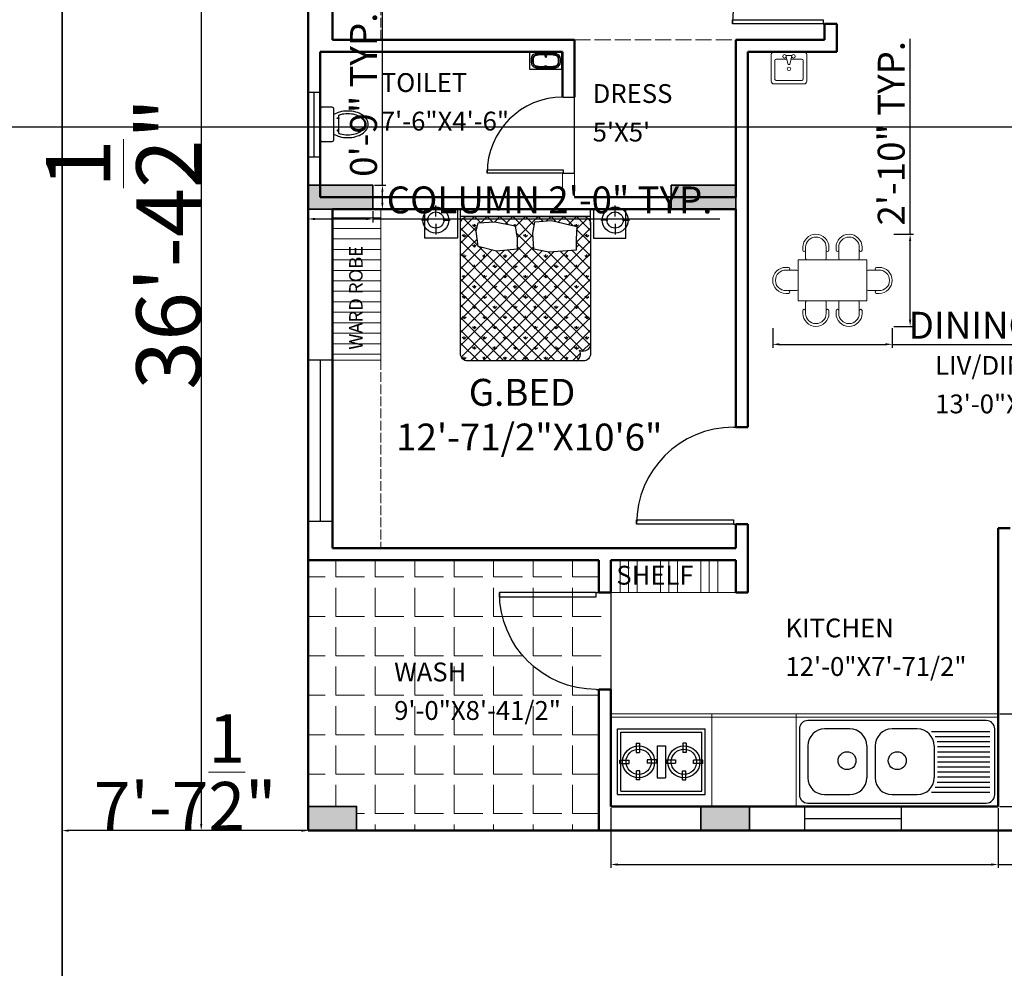
# Model space of a CAD drawing. Units: inches. Extents: x 2214 to 3937, y 762 to 2085.
# Tile 3 of 9: x 2567 to 2933, y 1424 to 1777. Entities that reach past the tile are written whole.
import ezdxf

# ---------------------------------------------------------------- set-up
doc = ezdxf.new("R2010")
doc.units = ezdxf.units.IN
doc.linetypes.add('ACAD_ISO02W100', pattern=[15, 12, -3])
for name, color, linetype, lineweight in [('A-ANNO-DIMS', 2, 'Continuous', 18), ('A-ANNO-TEXT', 7, 'Continuous', 18), ('A-AREA-IDEN', 7, 'Continuous', 25), ('A-CASE', 252, 'Continuous', 18), ('A-CASE-OVHD', 252, 'ACAD_ISO02W100', 13), ('A-CASE-PATT', 252, 'Continuous', 13), ('A-COLS', 5, 'Continuous', 35), ('A-FLOR-FIXT', 9, 'Continuous', 18), ('A-FLOR-PATT', 116, 'Continuous', 13), ('A-FURN', 8, 'Continuous', 18), ('A-WALL-OVHD', 20, 'ACAD_ISO02W100', 18), ('C-ANNO-DIMS', 2, 'Continuous', 18), ('C-PROP', 3, 'Continuous', 35), ('door', 122, 'Continuous', 25), ('wall', 20, 'Continuous', 50), ('wardrobe', 252, 'Continuous', 18), ('window', 4, 'Continuous', 25)]:
    doc.layers.add(name, color=color, linetype=linetype, lineweight=lineweight)
for name, color, linetype in [('GIUONG', 70, 'Continuous'), ('NOI THAT', 42, 'Continuous'), ('THIET-BI', 21, 'Continuous')]:
    doc.layers.add(name, color=color, linetype=linetype)
doc.styles.add('ATT', font='romans.shx')
doc.styles.get("Standard").update_dxf_attribs({"font": 'arial.ttf'})
doc.dimstyles.new('ISO-25', dxfattribs={"dimtxt": 10, "dimasz": 2.5, "dimexe": 1.25, "dimexo": 0.625, "dimtad": 1, "dimdec": 1, "dimlunit": 4, "dimtxsty": 'Standard', "dimcen": 2.5, "dimadec": 0, "dimazin": 0, "dimtfac": 1, "dimtdec": 1, "dimtmove": 0, "dimatfit": 3, "dimfxl": 1, "dimarcsym": 0})

# ---------------------------------------------------------------- blocks, each defined once
blk = doc.blocks.new('*U2')
for p, q in [((0, 0), (0, -6)), ((40, 0), (40, -6))]:
    blk.add_line(p, q)
blk.add_lwpolyline([(0, 0), (0, 40), (1.75, 40), (1.75, 0)], close=True)
blk.add_arc((0, 0), 40, 0, 90)
blk = doc.blocks.new('A$C65B13726')
at = {"layer": 'THIET-BI'}
for p, q in [((0, 400), (0, 200)), ((0, 400), (375, 400)), ((134, 362), (621, 360)), ((375, 291), (357, 291)), ((357, 291), (393, 291)), ((375, 291), (375, 309)), ((375, 309), (375, 274)), ((134, 39), (616, 39))]:
    blk.add_line(p, q, dxfattribs=at)
blk.add_lwpolyline([(0, 400), (0, 0), (750, 0), (750, 400)], close=True, dxfattribs=at)
blk.add_lwpolyline([(714, 200), (714, 240, 0.341607), (621, 360), (598, 366, 0.001439), (593, 367, 0.035276), (375, 382, 0.035276), (157, 367, 0.001439), (152, 366), (129, 360, 0.341607), (36, 240), (36, 200), (36, 161, 0.341607), (129, 40), (152, 34, 0.001439), (157, 33, 0.035276), (375, 18, 0.035276), (593, 33, 0.001439), (598, 34), (621, 40, 0.341607), (714, 161)], format="xyb", close=True, dxfattribs=at)
for points in [[(323, 348, 0.026733), (162, 334, 0.000876), (159, 333), (137, 327, 0.341782), (70, 240), (70, 161, 0.341782), (137, 73), (159, 67, 0.000876), (162, 67, 0.026747), (323, 52, 0.035276)], [(337, 337, 0.028876), (163, 323, 0.00069), (161, 322), (140, 317, 0.341861), (81, 240), (81, 160, 0.341861), (140, 83), (161, 78, 0.00069), (163, 77, 0.028898), (337, 63, 0.035276)], [(407, 348, 0.00526), (375, 349, 0.005313), (343, 348, 0.000876)], [(394, 338, 0.003179), (375, 338, 0.003179), (356, 338, 0.00069)], [(375, 382), (375, 382, 0.025118)], [(375, 382), (375, 382, 0.035276)], [(669, 200), (669, 240, 0.341861), (610, 317), (589, 322, 0.00069), (587, 323, 0.028876), (413, 337, 0.003179)], [(680, 200), (680, 240, 0.341782), (613, 327), (591, 333, 0.000876), (588, 334, 0.026733), (427, 348, 0.006503)], [(343, 52, 0.005316), (375, 52, 0.005263), (407, 52, 0.000876)], [(356, 62, 0.003135), (375, 62, 0.003135), (394, 62, 0.00069)], [(375, 17), (375, 17, 0.035276)], [(413, 63, 0.028961), (587, 77, 0.00069), (589, 78), (610, 83, 0.341861), (669, 160), (669, 200)], [(427, 52, 0.026747), (588, 67, 0.000876), (591, 67), (613, 73, 0.341782), (680, 161), (680, 200)]]:
    blk.add_lwpolyline(points, format="xyb", dxfattribs=at)
blk.add_circle((375, 291), 14.5, dxfattribs=at)
for centre, radius, start, end in [((375, 400), 73.6, 211.9576, 327.7237), ((324, 352), 19.1, 310.8832, 28.9258), ((375, 400), 65.2, 239.0852, 300.5961), ((426, 351), 19.1, 150.7555, 228.798), ((375, 0), 73.6, 32.2763, 148.0424), ((324, 48), 19.1, 331.0742, 49.1168), ((375, 0), 65.2, 59.4039, 120.9148), ((426, 49), 19.1, 131.202, 209.2445)]:
    blk.add_arc(centre, radius, start, end, dxfattribs=at)
blk = doc.blocks.new('A$C5AF77858')
at = {"layer": 'THIET-BI'}
for p, q in [((0, 675), (0, 525)), ((475, 700), (25, 700)), ((500, 525), (500, 675)), ((25, 500), (475, 500)), ((154, 452), (154, 430)), ((164, 452), (154, 452)), ((164, 430), (164, 452)), ((336, 430), (336, 452)), ((336, 452), (346, 452)), ((346, 452), (346, 430)), ((117, 430), (383, 430)), ((154, 430), (164, 430)), ((346, 430), (336, 430))]:
    blk.add_line(p, q, dxfattribs=at)
for centre, radius, start, end in [((25, 675), 25, 90, 180), ((475, 675), 25, 0, 90), ((25, 525), 25, 180, 270), ((384, 334), 323, 149.0966, 164.9269), ((116, 334), 323, 15.0731, 30.9034), ((475, 525), 25, 270, 0), ((514, 299), 458, 164.9269, 180), ((514, 299), 458, 180, 195.0731), ((514, 299), 418, 164.9269, 180), ((514, 299), 418, 180, 195.0731), ((384, 334), 283, 160.176, 164.9269), ((116, 334), 283, 15.0731, 19.824), ((-14, 299), 418, 0, 15.0731), ((-14, 299), 418, 344.9269, 0), ((-14, 299), 458, 0, 15.0731), ((-14, 299), 458, 344.9269, 0), ((384, 264), 323, 195.0731, 213.0315), ((384, 264), 283, 195.0731, 213.0315), ((116, 264), 283, 326.9685, 344.9269), ((116, 264), 323, 326.9685, 344.9269), ((302, 210), 226, 213.0315, 237.5002), ((302, 210), 186, 213.0315, 237.5002), ((250, 129), 129, 237.5002, 270), ((250, 129), 89.3, 237.5002, 270), ((250, 129), 89.3, 270, 302.4998), ((250, 129), 129, 270, 302.4998), ((198, 210), 186, 302.4998, 326.9685), ((198, 210), 226, 302.4998, 326.9685)]:
    blk.add_arc(centre, radius, start, end, dxfattribs=at)
blk = doc.blocks.new('*X8')
at = {"color": 0}
for p, q in [((0, 0), (0, 0)), ((-707, -141), (-734, -115)), ((-707, -141), (-707, -104)), ((-707, -141), (-681, -115)), ((-566, 0), (-566, 0)), ((-566, 0), (-566, 0)), ((-283, 0), (-283, 0)), ((-283, 0), (-283, 0)), ((-156, -126), (-168, -115)), ((-141, -141), (-141, -104)), ((-141, -141), (-115, -115)), ((120, -120), (115, -115)), ((283, 0), (283, 0)), ((566, 0), (566, 0)), ((699, -134), (681, -115)), ((707, -135), (707, -104)), ((710, -139), (734, -115)), ((-849, -283), (-875, -256)), ((-849, -283), (-849, -245)), ((-849, -283), (-822, -256)), ((-141, -141), (-142, -140)), ((0, -283), (-27, -256)), ((0, -283), (0, -245)), ((0, -283), (27, -256)), ((849, -283), (822, -256)), ((849, -283), (849, -245)), ((849, -283), (875, -256)), ((-707, -424), (-734, -398)), ((-707, -424), (-707, -387)), ((-707, -424), (-681, -398)), ((-116, -399), (-115, -398)), ((707, -424), (707, -387)), ((707, -424), (734, -398)), ((-849, -566), (-875, -539)), ((-849, -566), (-849, -528)), ((-849, -566), (-822, -539)), ((-566, -566), (-592, -539)), ((-566, -566), (-566, -528)), ((-566, -566), (-539, -539)), ((-283, -566), (-309, -539)), ((-283, -566), (-283, -528)), ((-283, -566), (-256, -539)), ((0, -566), (-27, -539)), ((0, -566), (0, -528)), ((0, -566), (27, -539)), ((283, -566), (256, -539)), ((283, -566), (283, -528)), ((283, -566), (309, -539)), ((566, -566), (539, -539)), ((566, -566), (566, -528)), ((566, -566), (592, -539)), ((707, -424), (703, -420)), ((849, -566), (822, -539)), ((849, -566), (849, -528)), ((849, -566), (875, -539)), ((-707, -707), (-734, -681)), ((-707, -707), (-707, -670)), ((-707, -707), (-681, -681)), ((-424, -707), (-451, -681)), ((-424, -707), (-424, -670)), ((-424, -707), (-398, -681)), ((-141, -707), (-168, -681)), ((-141, -707), (-141, -670)), ((-141, -707), (-115, -681)), ((141, -707), (115, -681)), ((141, -707), (141, -670)), ((141, -707), (168, -681)), ((424, -707), (398, -681)), ((424, -707), (424, -670)), ((424, -707), (451, -681)), ((707, -707), (681, -681)), ((707, -707), (707, -670)), ((707, -707), (734, -681)), ((-849, -849), (-849, -811)), ((-566, -849), (-566, -811)), ((-283, -849), (-283, -811)), ((0, -849), (0, -811)), ((283, -849), (283, -811)), ((566, -849), (566, -811)), ((849, -849), (849, -811)), ((-849, -849), (-875, -822)), ((-849, -849), (-822, -822)), ((-707, -990), (-707, -952)), ((-566, -849), (-592, -822)), ((-566, -849), (-539, -822)), ((-424, -990), (-424, -952)), ((-283, -849), (-309, -822)), ((-283, -849), (-256, -822)), ((-141, -990), (-141, -952)), ((0, -849), (-27, -822)), ((0, -849), (27, -822)), ((141, -990), (141, -952)), ((283, -849), (256, -822)), ((283, -849), (309, -822)), ((424, -990), (424, -952)), ((566, -849), (539, -822)), ((566, -849), (592, -822)), ((707, -990), (707, -952)), ((849, -849), (822, -822)), ((849, -849), (875, -822)), ((-707, -990), (-734, -963)), ((-707, -990), (-681, -963)), ((-424, -990), (-451, -963)), ((-424, -990), (-398, -963)), ((-141, -990), (-168, -963)), ((-141, -990), (-115, -963)), ((141, -990), (115, -963)), ((141, -990), (168, -963)), ((424, -990), (398, -963)), ((424, -990), (451, -963)), ((707, -990), (681, -963)), ((707, -990), (734, -963)), ((-849, -1131), (-875, -1105)), ((-849, -1131), (-849, -1094)), ((-849, -1131), (-822, -1105)), ((-566, -1131), (-592, -1105)), ((-566, -1131), (-566, -1094)), ((-566, -1131), (-539, -1105)), ((-283, -1131), (-309, -1105)), ((-283, -1131), (-283, -1094)), ((-283, -1131), (-256, -1105)), ((0, -1131), (-27, -1105)), ((0, -1131), (0, -1094)), ((0, -1131), (27, -1105)), ((283, -1131), (256, -1105)), ((283, -1131), (283, -1094)), ((283, -1131), (309, -1105)), ((566, -1131), (539, -1105)), ((566, -1131), (566, -1094)), ((566, -1131), (592, -1105)), ((849, -1131), (822, -1105)), ((849, -1131), (849, -1094)), ((849, -1131), (875, -1105)), ((-707, -1273), (-734, -1246)), ((-707, -1273), (-707, -1235)), ((-707, -1273), (-681, -1246)), ((-424, -1273), (-451, -1246)), ((-424, -1273), (-424, -1235)), ((-424, -1273), (-398, -1246)), ((-141, -1273), (-168, -1246)), ((-141, -1273), (-141, -1235)), ((-141, -1273), (-115, -1246)), ((141, -1273), (115, -1246)), ((141, -1273), (141, -1235)), ((141, -1273), (168, -1246)), ((424, -1273), (398, -1246)), ((424, -1273), (424, -1235)), ((424, -1273), (451, -1246)), ((707, -1273), (681, -1246)), ((707, -1273), (707, -1235)), ((707, -1273), (734, -1246)), ((-849, -1414), (-875, -1388)), ((-849, -1414), (-849, -1377)), ((-849, -1414), (-822, -1388)), ((-566, -1414), (-592, -1388)), ((-566, -1414), (-566, -1377)), ((-566, -1414), (-539, -1388)), ((-283, -1414), (-309, -1388)), ((-283, -1414), (-283, -1377)), ((-283, -1414), (-256, -1388)), ((0, -1414), (-27, -1388)), ((0, -1414), (0, -1377)), ((0, -1414), (27, -1388)), ((283, -1414), (256, -1388)), ((283, -1414), (283, -1377)), ((283, -1414), (309, -1388)), ((566, -1414), (539, -1388)), ((566, -1414), (566, -1377)), ((566, -1414), (592, -1388)), ((849, -1414), (822, -1388)), ((849, -1414), (849, -1377)), ((849, -1414), (875, -1388)), ((-707, -1556), (-734, -1529)), ((-707, -1556), (-707, -1518)), ((-707, -1556), (-681, -1529)), ((-424, -1556), (-451, -1529)), ((-424, -1556), (-424, -1518)), ((-424, -1556), (-398, -1529)), ((-141, -1556), (-168, -1529)), ((-141, -1556), (-141, -1518)), ((-141, -1556), (-115, -1529)), ((141, -1556), (115, -1529)), ((141, -1556), (141, -1518)), ((141, -1556), (168, -1529)), ((424, -1556), (398, -1529)), ((424, -1556), (424, -1518)), ((424, -1556), (451, -1529)), ((707, -1556), (681, -1529)), ((707, -1556), (707, -1518)), ((707, -1556), (734, -1529)), ((-849, -1697), (-875, -1671)), ((-849, -1697), (-849, -1660)), ((-849, -1697), (-822, -1671)), ((-566, -1697), (-592, -1671)), ((-566, -1697), (-566, -1660)), ((-566, -1697), (-539, -1671)), ((-283, -1697), (-309, -1671)), ((-283, -1697), (-283, -1660)), ((-283, -1697), (-256, -1671)), ((0, -1697), (-27, -1671)), ((0, -1697), (0, -1660)), ((0, -1697), (27, -1671)), ((283, -1697), (256, -1671)), ((283, -1697), (283, -1660)), ((283, -1697), (309, -1671)), ((566, -1697), (539, -1671)), ((566, -1697), (566, -1660)), ((566, -1697), (592, -1671)), ((849, -1697), (822, -1671)), ((849, -1697), (849, -1660)), ((849, -1697), (875, -1671)), ((-707, -1838), (-734, -1812)), ((-707, -1838), (-707, -1801)), ((-707, -1838), (-681, -1812)), ((-424, -1838), (-451, -1812)), ((-424, -1838), (-424, -1801)), ((-424, -1838), (-398, -1812)), ((-141, -1838), (-168, -1812)), ((-141, -1838), (-141, -1801)), ((-141, -1838), (-115, -1812)), ((141, -1838), (115, -1812)), ((141, -1838), (141, -1801)), ((141, -1838), (168, -1812)), ((424, -1838), (398, -1812)), ((424, -1838), (424, -1801)), ((424, -1838), (451, -1812)), ((707, -1838), (681, -1812)), ((707, -1838), (707, -1801)), ((707, -1838), (734, -1812)), ((-849, -1980), (-875, -1953)), ((-849, -1980), (-849, -1942)), ((-849, -1980), (-822, -1953)), ((-566, -1980), (-592, -1953)), ((-566, -1980), (-566, -1942)), ((-566, -1980), (-539, -1953)), ((-283, -1980), (-309, -1953)), ((-283, -1980), (-283, -1942)), ((-283, -1980), (-256, -1953)), ((0, -1980), (-27, -1953)), ((0, -1980), (0, -1942)), ((0, -1980), (27, -1953)), ((283, -1980), (256, -1953)), ((283, -1980), (283, -1942)), ((283, -1980), (309, -1953)), ((566, -1980), (539, -1953)), ((566, -1980), (566, -1942)), ((566, -1980), (592, -1953))]:
    blk.add_line(p, q, dxfattribs=at)
blk = doc.blocks.new('*X7')
at = {"color": 0}
for p, q in [((-900, -193), (-707, 0)), ((-623, -84), (-707, 0)), ((-614, -83), (-530, 0)), ((-457, -74), (-530, 0)), ((-425, -72), (-354, 0)), ((-245, -108), (-354, 0)), ((-278, -101), (-177, 0)), ((103, -280), (-177, 0)), ((-142, -142), (0, 0)), ((-117, -294), (177, 0)), ((120, -120), (0, 0)), ((241, -64), (177, 0)), ((292, -61), (354, 0)), ((426, -72), (354, 0)), ((452, -78), (530, 0)), ((654, -123), (530, 0)), ((596, -111), (707, 0)), ((900, -193), (707, 0)), ((-683, -201), (-862, -22)), ((708, -175), (862, -22)), ((-900, -370), (-667, -137)), ((-656, -405), (-900, -161)), ((-900, -1254), (101, -252)), ((900, -1254), (-128, -225)), ((703, -358), (900, -161)), ((900, -370), (708, -178)), ((-900, -546), (-668, -314)), ((735, -1973), (-900, -337)), ((-763, -2000), (900, -337)), ((900, -546), (703, -349)), ((-900, -1430), (112, -418)), ((-900, -723), (-605, -429)), ((-900, -900), (-465, -465)), ((-900, -1077), (-293, -470)), ((-900, -1607), (231, -476)), ((-900, -1784), (394, -489)), ((586, -2000), (-900, -514)), ((-888, -1948), (586, -475)), ((801, -1862), (-641, -419)), ((-586, -2000), (900, -514)), ((900, -1784), (-404, -480)), ((900, -1607), (-243, -465)), ((900, -1430), (-116, -415)), ((900, -1077), (317, -494)), ((900, -900), (483, -483)), ((900, -723), (647, -470)), ((409, -2000), (-900, -691)), ((-409, -2000), (900, -691)), ((232, -2000), (-900, -868)), ((-232, -2000), (900, -868)), ((55, -2000), (-900, -1045)), ((-55, -2000), (900, -1045)), ((-121, -2000), (-900, -1221)), ((121, -2000), (900, -1221)), ((-298, -2000), (-900, -1398)), ((298, -2000), (900, -1398)), ((-475, -2000), (-900, -1575)), ((475, -2000), (900, -1575)), ((-652, -2000), (-900, -1752)), ((790, -1861), (900, -1752)), ((652, -2000), (761, -1890)), ((-835, -1994), (-894, -1935))]:
    blk.add_line(p, q, dxfattribs=at)
blk = doc.blocks.new('A$C190D2546')
at = {"layer": 'GIUONG'}
for points in [[(787, 1584), (758, 1799), (787, 1914), (1016, 1928), (1296, 1871), (1325, 1699), (1325, 1548), (1038, 1519)], [(1555, 1548), (1541, 1771), (1569, 1928), (1799, 1943), (2151, 1864), (2144, 1685), (2144, 1534), (1763, 1505)]]:
    blk.add_lwpolyline(points, close=True, dxfattribs=at)
for centre, radius in [((200, 1951), 180), ((200, 1951), 112), ((2682, 1951), 180), ((2682, 1951), 112)]:
    blk.add_circle(centre, radius, dxfattribs=at)
at = {"layer": 'NOI THAT'}
for p, q in [((200, 2001), (200, 2151)), ((541, 2100), (2341, 2100)), ((541, 1881), (541, 2100)), ((2341, 1881), (2341, 2100)), ((2682, 2001), (2682, 2151)), ((100, 1951), (0, 1951)), ((300, 1951), (400, 1951)), ((2341, 2000), (541, 2000)), ((2582, 1951), (2482, 1951)), ((2782, 1951), (2882, 1951)), ((200, 1901), (200, 1751)), ((2682, 1901), (2682, 1751))]:
    blk.add_line(p, q, dxfattribs=at)
for points in [[(500, 2101), (500, 1701), (50, 1701), (50, 2101)], [(2382, 2101), (2382, 1701), (2832, 1701), (2832, 2101)]]:
    blk.add_lwpolyline(points, close=True, dxfattribs=at)
blk.add_lwpolyline([(641, 2000), (2241, 2000, -0.414214), (2341, 1900), (2341, 100, -0.414214), (2241, 0), (641, 0, -0.414214), (541, 100), (541, 1900, -0.414214)], format="xyb", close=True, dxfattribs=at)
for centre, start, end in [((2091, 100), 296.5651, 26.5651), ((2241, 250), 243.4349, 333.4349)]:
    blk.add_arc(centre, 112, start, end, dxfattribs=at)
for name in ['*X7', '*X8']:
    blk.add_blockref(name, (1441, 2000), dxfattribs=at)
blk = doc.blocks.new('A$C5AA626B0')
for p, q in [((661, 1672), (661, 1732)), ((721, 1488), (721, 1732)), ((1171, 1732), (1171, 1488)), ((1231, 1732), (1231, 1672)), ((1386, 1732), (1386, 1672)), ((1446, 1732), (1446, 1488)), ((1896, 1488), (1896, 1732)), ((1956, 1672), (1956, 1732)), ((558, 1458), (2058, 1458)), ((558, 558), (558, 1458)), ((1476, 1458), (1866, 1458)), ((2058, 1458), (2058, 558)), ((285, 1293), (345, 1293)), ((285, 1233), (528, 1233)), ((558, 1203), (558, 813)), ((2058, 813), (2058, 1203)), ((2088, 1233), (2332, 1233)), ((2272, 1293), (2332, 1293)), ((528, 783), (285, 783)), ((345, 723), (285, 723)), ((2332, 783), (2088, 783)), ((2332, 723), (2272, 723)), ((2058, 558), (558, 558)), ((721, 528), (721, 285)), ((1171, 285), (1171, 528)), ((1446, 285), (1446, 528)), ((1476, 558), (1866, 558)), ((1896, 528), (1896, 285)), ((661, 345), (661, 285)), ((1231, 285), (1231, 345)), ((1386, 285), (1386, 345)), ((1956, 345), (1956, 285))]:
    blk.add_line(p, q)
for centre, radius, start, end in [((946, 1732), 285, 0, 180), ((946, 1732), 225, 0, 180), ((1671, 1732), 285, 0, 180), ((1671, 1732), 225, 0, 180), ((691, 1672), 30, 180, 0), ((1201, 1672), 30, 180, 0), ((1416, 1672), 30, 180, 0), ((1926, 1672), 30, 180, 0), ((751, 1488), 30, 180, 270), ((1141, 1488), 30, 270, 0), ((1476, 1488), 30, 180, 270), ((1866, 1488), 30, 270, 0), ((285, 1008), 285, 90, 270), ((285, 1008), 225, 90, 270), ((345, 1263), 30, 270, 90), ((528, 1203), 30, 0, 90), ((2088, 1203), 30, 90, 180), ((2272, 1263), 30, 90, 270), ((2332, 1008), 285, 270, 90), ((2332, 1008), 225, 270, 90), ((345, 753), 30, 270, 90), ((528, 813), 30, 270, 0), ((2088, 813), 30, 180, 270), ((2272, 753), 30, 90, 270), ((751, 528), 30, 90, 180), ((1141, 528), 30, 0, 90), ((1476, 528), 30, 90, 180), ((1866, 528), 30, 0, 90), ((691, 345), 30, 0, 180), ((946, 285), 285, 180, 0), ((946, 285), 225, 180, 0), ((1201, 345), 30, 0, 180), ((1416, 345), 30, 0, 180), ((1671, 285), 285, 180, 0), ((1671, 285), 225, 180, 0), ((1926, 345), 30, 0, 180)]:
    blk.add_arc(centre, radius, start, end)
blk = doc.blocks.new('15PLAV06')
at = {"color": 0, "linetype": 'ByBlock'}
for p, q in [((0, 8.5), (0, -8.5)), ((16.5, 10), (1.5, 10)), ((4, 1.25), (4, 7.25)), ((4.75, 8), (15.25, 8)), ((16, 7.25), (16, -7.25)), ((18, -8.5), (18, 8.5)), ((2, -1.5), (2, 1.5)), ((7, 0.5), (3, 1.5)), ((7, -0.5), (7, 0.5)), ((3, -1.5), (7, -0.5)), ((4, -7.25), (4, -1.25)), ((1.5, -10), (16.5, -10)), ((15.25, -8), (4.75, -8))]:
    blk.add_line(p, q, dxfattribs=at)
for centre in [(2.5, 2.5), (9.5, 0), (2.5, -2.5)]:
    blk.add_circle(centre, 1, dxfattribs=at)
for centre, radius, start, end in [((1.5, 8.5), 1.5, 90, 180), ((4.75, 7.25), 0.75, 90, 180), ((15.25, 7.25), 0.75, 0, 90), ((16.5, 8.5), 1.5, 0, 90), ((1.5, -8.5), 1.5, 180, 270), ((4.75, -7.25), 0.75, 180, 270), ((15.25, -7.25), 0.75, 270, 0), ((16.5, -8.5), 1.5, 270, 0)]:
    blk.add_arc(centre, radius, start, end, dxfattribs=at)
at = {"color": 0, "linetype": 'ByBlock', "style": 'ATT'}
for tag, p, flags in [('ITEM', (0, -20), 3), ('ROOM_NUMBER', (0, -29), 1)]:
    blk.add_attdef(tag, p, '', height=6, dxfattribs=dict(at, flags=flags))
blk = doc.blocks.new('A$C1D6C0704')
for p, q in [((0, 550), (2300, 550)), ((0, 0), (0, 550)), ((0, 530), (2300, 530)), ((600, 0), (600, 550)), ((1100, 0), (1100, 550)), ((2300, 550), (2300, 0)), ((2300, 0), (0, 0))]:
    blk.add_line(p, q)
at = {"layer": 'NOI THAT'}
for p, q in [((2230, 510), (1170, 510)), ((40, 70), (40, 460)), ((40, 460), (560, 460)), ((60, 90), (60, 440)), ((60, 440), (540, 440)), ((540, 90), (540, 440)), ((560, 70), (560, 460)), ((1120, 460), (1120, 70)), ((1420, 460), (1270, 460)), ((1820, 460), (1670, 460)), ((1904.7, 445), (2250, 445)), ((1926.7, 415), (2250, 415)), ((2280, 70), (2280, 460)), ((151.4, 375), (151.4, 320)), ((151.4, 375), (171.4, 375)), ((171.4, 375), (171.4, 320)), ((275, 360), (325, 360)), ((275, 360), (275, 170)), ((325, 360), (325, 170)), ((448.6, 375), (428.6, 375)), ((428.6, 375), (428.6, 320)), ((448.6, 375), (448.6, 320)), ((1170, 360), (1170, 170)), ((1520, 360), (1520, 170)), ((1570, 360), (1570, 170)), ((1920, 360), (1920, 170)), ((1937.4, 385), (2250, 385)), ((1940, 355), (2250, 355)), ((151.4, 320), (171.4, 320)), ((448.6, 320), (428.6, 320)), ((1940, 325), (2250, 325)), ((1940, 295), (2250, 295)), ((53.4, 255), (53.4, 275)), ((53.4, 275), (108.4, 275)), ((53.4, 255), (108.4, 255)), ((108.4, 255), (108.4, 275)), ((271.4, 277), (216.4, 277)), ((216.4, 277), (216.4, 257)), ((271.4, 257), (216.4, 257)), ((271.4, 277), (271.4, 257)), ((328.6, 277), (383.6, 277)), ((328.6, 277), (328.6, 257)), ((328.6, 257), (383.6, 257)), ((383.6, 277), (383.6, 257)), ((491.6, 255), (491.6, 275)), ((546.6, 275), (491.6, 275)), ((546.6, 255), (491.6, 255)), ((546.6, 255), (546.6, 275)), ((1940, 265), (2250, 265)), ((1940, 235), (2250, 235)), ((153.4, 157), (153.4, 212)), ((173.4, 212), (153.4, 212)), ((173.4, 157), (173.4, 212)), ((426.6, 157), (426.6, 212)), ((426.6, 212), (446.6, 212)), ((446.6, 157), (446.6, 212)), ((1940, 205), (2250, 205)), ((173.4, 157), (153.4, 157)), ((275, 170), (325, 170)), ((426.6, 157), (446.6, 157)), ((1937.4, 145), (2250, 145)), ((1940, 175), (2250, 175)), ((40, 70), (560, 70)), ((60, 90), (540, 90)), ((1270, 70), (1420, 70)), ((1670, 70), (1820, 70)), ((1904.7, 85), (2250, 85)), ((1926.7, 115), (2250, 115)), ((1170, 20), (2230, 20))]:
    blk.add_line(p, q, dxfattribs=at)
for centre, radius in [((165.5, 265.1), 95), ((434.5, 265.1), 95), ((165.5, 265.1), 75), ((434.5, 265.1), 75), ((1402.9, 271.7), 53.2), ((1701.1, 271.7), 53.2)]:
    blk.add_circle(centre, radius, dxfattribs=at)
for centre, radius, start, end in [((1170, 460), 50, 90, 180), ((2230, 460), 50, 0, 90), ((1270, 360), 100, 90, 180), ((1420, 360), 100, 0, 90), ((1670, 360), 100, 90, 180), ((1820, 360), 100, 0, 90), ((1270, 170), 100, 180, 270), ((1420, 170), 100, 270, 0), ((1670, 170), 100, 180, 270), ((1820, 170), 100, 270, 0), ((1170, 70), 50, 180, 270), ((2230, 70), 50, 270, 0)]:
    blk.add_arc(centre, radius, start, end, dxfattribs=at)
blk = doc.blocks.new('*D18')
at = {"layer": 'A-ANNO-DIMS', "color": 0, "lineweight": -2, "ltscale": 0.3, "transparency": 16777216}
for p, q in [((2673.43, 1911.72), (2633.05, 1911.72)), ((2634.3, 1909.22), (2634.3, 1477.72)), ((2673.43, 1475.22), (2633.05, 1475.22))]:
    blk.add_line(p, q, dxfattribs=at)
at = {"layer": 'A-ANNO-DIMS', "color": 0, "ltscale": 0.3, "transparency": 16777216}
for points in [[(2633.89, 1909.22), (2634.72, 1909.22), (2634.3, 1911.72)], [(2633.89, 1477.72), (2634.72, 1477.72), (2634.3, 1475.22)]]:
    blk.add_solid(points, dxfattribs=at)
at = {"layer": 'Defpoints', "color": 0, "ltscale": 0.3, "transparency": 16777216}
for p in [(2674.06, 1911.72), (2634.3, 1475.22), (2674.06, 1475.22)]:
    blk.add_point(p, dxfattribs=at)
at = {"layer": 'A-ANNO-DIMS', "color": 0, "ltscale": 0.3, "transparency": 16777216, "insert": (2605.37, 1693.47), "char_height": 24, "attachment_point": 5, "rotation": 90}
blk.add_mtext('36\'-4{\\H1x;\\S1/2;}"', dxfattribs=at)
blk = doc.blocks.new('*D20')
at = {"layer": 'C-ANNO-DIMS', "color": 0, "lineweight": -2, "ltscale": 0.3, "transparency": 16777216}
for p, q in [((2581.93, 2003.22), (2545.31, 2003.22)), ((2546.56, 2000.72), (2546.56, 1357.72)), ((2581.93, 1355.22), (2545.31, 1355.22))]:
    blk.add_line(p, q, dxfattribs=at)
at = {"layer": 'C-ANNO-DIMS', "color": 0, "ltscale": 0.3, "transparency": 16777216}
for points in [[(2546.14, 2000.72), (2546.97, 2000.72), (2546.56, 2003.22)], [(2546.14, 1357.72), (2546.97, 1357.72), (2546.56, 1355.22)]]:
    blk.add_solid(points, dxfattribs=at)
at = {"layer": 'Defpoints', "color": 0, "ltscale": 0.3, "transparency": 16777216}
for p in [(2582.56, 2003.22), (2546.56, 1355.22), (2582.56, 1355.22)]:
    blk.add_point(p, dxfattribs=at)
at = {"layer": 'C-ANNO-DIMS', "color": 0, "ltscale": 0.3, "transparency": 16777216, "insert": (2533.73, 1679.22), "char_height": 24, "attachment_point": 5, "rotation": 90}
blk.add_mtext("54'", dxfattribs=at)
blk = doc.blocks.new('*D24')
at = {"layer": 'C-ANNO-DIMS', "color": 0, "lineweight": -2, "ltscale": 0.3, "transparency": 16777216}
for p, q in [((2582.56, 1475.84), (2582.56, 1476.47)), ((2671.56, 1475.22), (2585.06, 1475.22)), ((2674.06, 1475.84), (2674.06, 1476.47))]:
    blk.add_line(p, q, dxfattribs=at)
at = {"layer": 'C-ANNO-DIMS', "color": 0, "ltscale": 0.3, "transparency": 16777216}
for points in [[(2585.06, 1475.64), (2585.06, 1474.8), (2582.56, 1475.22)], [(2671.56, 1475.64), (2671.56, 1474.8), (2674.06, 1475.22)]]:
    blk.add_solid(points, dxfattribs=at)
at = {"layer": 'Defpoints', "color": 0, "ltscale": 0.3, "transparency": 16777216}
for p in [(2582.56, 1475.22), (2582.56, 1475.22), (2674.06, 1475.22)]:
    blk.add_point(p, dxfattribs=at)
at = {"layer": 'C-ANNO-DIMS', "color": 0, "ltscale": 0.3, "transparency": 16777216, "insert": (2628.31, 1496.92), "char_height": 18, "attachment_point": 5}
blk.add_mtext('7\'-7{\\H1x;\\S1/2;}"', dxfattribs=at)
blk = doc.blocks.new('COL-18X9')
at = {"ltscale": 0.3}
h = blk.add_hatch(color=256, dxfattribs=at)
h.dxf.hatch_style = 1
h.paths.add_polyline_path([(18, 0), (18, 9), (0, 9), (0, 0)])
blk.add_lwpolyline([(0, 9), (18, 9), (18, 0), (0, 0)], close=True, dxfattribs=at)
blk = doc.blocks.new('COL-24X9')
at = {"ltscale": 0.3}
h = blk.add_hatch(color=256, dxfattribs=at)
h.dxf.hatch_style = 1
h.paths.add_polyline_path([(24, 0), (24, 9), (0, 9), (0, 0)])
blk.add_line((24, 9), (24, 0))
blk.add_lwpolyline([(0, 9), (24, 9), (24, 0), (0, 0)], close=True, dxfattribs=at)
blk = doc.blocks.new('WIN-24X4_5')
for p, q in [((0, 0), (0, 4.5)), ((24, 0), (24, 4.5))]:
    blk.add_line(p, q)
at = {"ltscale": 0.3}
blk.add_line((24, 2.25), (0, 2.25), dxfattribs=at)
blk = doc.blocks.new('*D37')
at = {"layer": 'C-ANNO-DIMS', "color": 0, "lineweight": -2, "ltscale": 0.3, "transparency": 16777216}
for p, q in [((2674.06, 1705.59), (2674.06, 1701.37)), ((2676.56, 1702.62), (2695.56, 1702.62)), ((2698.06, 1705.59), (2698.06, 1701.37)), ((2698.06, 1702.62), (2827.07, 1702.62))]:
    blk.add_line(p, q, dxfattribs=at)
at = {"layer": 'C-ANNO-DIMS', "color": 0, "ltscale": 0.3, "transparency": 16777216}
for points in [[(2676.56, 1703.04), (2676.56, 1702.2), (2674.06, 1702.62)], [(2695.56, 1703.04), (2695.56, 1702.2), (2698.06, 1702.62)]]:
    blk.add_solid(points, dxfattribs=at)
at = {"layer": 'Defpoints', "color": 0, "ltscale": 0.3, "transparency": 16777216}
for p in [(2674.06, 1706.22), (2698.06, 1706.22), (2698.06, 1702.62)]:
    blk.add_point(p, dxfattribs=at)
at = {"layer": 'C-ANNO-DIMS', "color": 0, "ltscale": 0.3, "transparency": 16777216, "insert": (2763.81, 1708.42), "char_height": 10, "attachment_point": 5}
blk.add_mtext('COLUMN 2\'-0" TYP.', dxfattribs=at)
blk = doc.blocks.new('*D38')
at = {"layer": 'C-ANNO-DIMS', "color": 0, "lineweight": -2, "ltscale": 0.3, "transparency": 16777216}
for p, q in [((2701.66, 1715.22), (2701.66, 1779.92)), ((2698.68, 1715.22), (2702.91, 1715.22)), ((2701.66, 1708.72), (2701.66, 1712.72)), ((2698.68, 1706.22), (2702.91, 1706.22))]:
    blk.add_line(p, q, dxfattribs=at)
at = {"layer": 'C-ANNO-DIMS', "color": 0, "ltscale": 0.3, "transparency": 16777216}
for points in [[(2701.24, 1712.72), (2702.07, 1712.72), (2701.66, 1715.22)], [(2701.24, 1708.72), (2702.07, 1708.72), (2701.66, 1706.22)]]:
    blk.add_solid(points, dxfattribs=at)
at = {"layer": 'Defpoints', "color": 0, "ltscale": 0.3, "transparency": 16777216}
for p in [(2698.06, 1715.22), (2701.66, 1715.22), (2698.06, 1706.22)]:
    blk.add_point(p, dxfattribs=at)
at = {"layer": 'C-ANNO-DIMS', "color": 0, "ltscale": 0.3, "transparency": 16777216, "insert": (2695.93, 1748.82), "char_height": 10, "attachment_point": 5, "rotation": 90}
blk.add_mtext('0\'-9" TYP.', dxfattribs=at)
blk = doc.blocks.new('*D51')
at = {"layer": 'C-ANNO-DIMS', "color": 0, "lineweight": -2, "ltscale": 0.3, "transparency": 16777216}
for p, q in [((2846.77, 1662.06), (2846.77, 1654.77)), ((2891.18, 1662.06), (2891.18, 1654.77)), ((2849.27, 1656.02), (2888.68, 1656.02)), ((2891.18, 1656.02), (3062.52, 1656.02))]:
    blk.add_line(p, q, dxfattribs=at)
at = {"layer": 'C-ANNO-DIMS', "color": 0, "ltscale": 0.3, "transparency": 16777216}
for points in [[(2849.27, 1656.44), (2849.27, 1655.61), (2846.77, 1656.02)], [(2888.68, 1656.44), (2888.68, 1655.61), (2891.18, 1656.02)]]:
    blk.add_solid(points, dxfattribs=at)
at = {"layer": 'Defpoints', "color": 0, "ltscale": 0.3, "transparency": 16777216}
for p in [(2846.77, 1662.69), (2891.18, 1662.69), (2891.18, 1656.02)]:
    blk.add_point(p, dxfattribs=at)
at = {"layer": 'C-ANNO-DIMS', "color": 0, "ltscale": 0.3, "transparency": 16777216, "insert": (2978.1, 1661.82), "char_height": 10, "attachment_point": 5}
blk.add_mtext('DINING SET 3\'-8 1/2" TYP.', dxfattribs=at)
blk = doc.blocks.new('*D52')
at = {"layer": 'C-ANNO-DIMS', "color": 0, "lineweight": -2, "ltscale": 0.3, "transparency": 16777216}
for p, q in [((2897.84, 1696.92), (2897.84, 1769.56)), ((2891.81, 1696.92), (2899.09, 1696.92)), ((2897.84, 1665.19), (2897.84, 1694.42)), ((2891.81, 1662.69), (2899.09, 1662.69))]:
    blk.add_line(p, q, dxfattribs=at)
at = {"layer": 'C-ANNO-DIMS', "color": 0, "ltscale": 0.3, "transparency": 16777216}
for points in [[(2897.43, 1694.42), (2898.26, 1694.42), (2897.84, 1696.92)], [(2897.43, 1665.19), (2898.26, 1665.19), (2897.84, 1662.69)]]:
    blk.add_solid(points, dxfattribs=at)
at = {"layer": 'Defpoints', "color": 0, "ltscale": 0.3, "transparency": 16777216}
for p in [(2891.18, 1696.92), (2897.84, 1696.92), (2891.18, 1662.69)]:
    blk.add_point(p, dxfattribs=at)
at = {"layer": 'C-ANNO-DIMS', "color": 0, "ltscale": 0.3, "transparency": 16777216, "insert": (2892.11, 1734.49), "char_height": 10, "attachment_point": 5, "rotation": 90}
blk.add_mtext('2\'-10" TYP.', dxfattribs=at)
blk = doc.blocks.new('*D55')
at = {"layer": 'C-ANNO-DIMS', "color": 0, "lineweight": -2, "ltscale": 0.3, "transparency": 16777216}
for p, q in [((2786.56, 1483.59), (2786.56, 1461.37)), ((2930.56, 1483.59), (2930.56, 1461.37)), ((2789.06, 1462.62), (2928.06, 1462.62)), ((2930.56, 1462.62), (3106.37, 1462.62))]:
    blk.add_line(p, q, dxfattribs=at)
at = {"layer": 'C-ANNO-DIMS', "color": 0, "ltscale": 0.3, "transparency": 16777216}
for points in [[(2789.06, 1463.04), (2789.06, 1462.2), (2786.56, 1462.62)], [(2928.06, 1463.04), (2928.06, 1462.2), (2930.56, 1462.62)]]:
    blk.add_solid(points, dxfattribs=at)
at = {"layer": 'Defpoints', "color": 0, "ltscale": 0.3, "transparency": 16777216}
for p in [(2786.56, 1484.22), (2930.56, 1484.22), (2930.56, 1462.62)]:
    blk.add_point(p, dxfattribs=at)
at = {"layer": 'C-ANNO-DIMS', "color": 0, "ltscale": 0.3, "transparency": 16777216, "insert": (3019.71, 1468.42), "char_height": 10, "attachment_point": 5}
blk.add_mtext('KITCHEN COUNTER 12\'-0"', dxfattribs=at)
blk = doc.blocks.new('*D56')
at = {"layer": 'C-ANNO-DIMS', "color": 0, "lineweight": -2, "ltscale": 0.3, "transparency": 16777216}
for p, q in [((2952.16, 1518.65), (2952.16, 1580.23)), ((2931.18, 1518.65), (2953.41, 1518.65)), ((2952.16, 1486.72), (2952.16, 1516.15)), ((2931.18, 1484.22), (2953.41, 1484.22))]:
    blk.add_line(p, q, dxfattribs=at)
at = {"layer": 'C-ANNO-DIMS', "color": 0, "ltscale": 0.3, "transparency": 16777216}
for points in [[(2951.74, 1516.15), (2952.57, 1516.15), (2952.16, 1518.65)], [(2951.74, 1486.72), (2952.57, 1486.72), (2952.16, 1484.22)]]:
    blk.add_solid(points, dxfattribs=at)
at = {"layer": 'Defpoints', "color": 0, "ltscale": 0.3, "transparency": 16777216}
for p in [(2930.56, 1518.65), (2952.16, 1518.65), (2930.56, 1484.22)]:
    blk.add_point(p, dxfattribs=at)
at = {"layer": 'C-ANNO-DIMS', "color": 0, "ltscale": 0.3, "transparency": 16777216, "insert": (2946.36, 1550.69), "char_height": 10, "attachment_point": 5, "rotation": 90}
blk.add_mtext('2\'-10 1/2"', dxfattribs=at)
blk = doc.blocks.new('*D63')
at = {"layer": 'C-ANNO-DIMS', "color": 0, "lineweight": -2, "ltscale": 0.3, "transparency": 16777216}
for p, q in [((3240.43, 1875.72), (2225.23, 1875.72)), ((2226.48, 1873.22), (2226.48, 1739.22)), ((3240.43, 1736.72), (2225.23, 1736.72))]:
    blk.add_line(p, q, dxfattribs=at)
at = {"layer": 'C-ANNO-DIMS', "color": 0, "ltscale": 0.3, "transparency": 16777216}
for points in [[(2226.07, 1873.22), (2226.9, 1873.22), (2226.48, 1875.72)], [(2226.07, 1739.22), (2226.9, 1739.22), (2226.48, 1736.72)]]:
    blk.add_solid(points, dxfattribs=at)
at = {"layer": 'Defpoints', "color": 0, "ltscale": 0.3, "transparency": 16777216}
for p in [(3241.06, 1875.72), (2226.48, 1736.72), (3241.06, 1736.72)]:
    blk.add_point(p, dxfattribs=at)
at = {"layer": 'C-ANNO-DIMS', "color": 0, "ltscale": 0.3, "transparency": 16777216, "insert": (2220.84, 1806.22), "char_height": 10, "attachment_point": 5, "rotation": 90}
blk.add_mtext('11\'-7"', dxfattribs=at)

msp = doc.modelspace()

# ---------------------------------------------------------------- hatches: boundary and pattern name
at = {"layer": 'A-CASE-PATT', "ltscale": 0.3}
h = msp.add_hatch(dxfattribs=at)
h.set_pattern_fill('ANSI31', color=256, scale=1.227415, angle=-45, style=0)
h.paths.add_polyline_path([(2683.06, 1650.12), (2701.06, 1650.12), (2701.06, 1706.22), (2683.06, 1706.22)])
h = msp.add_hatch(dxfattribs=at)
h.set_pattern_fill('GOST_GROUND', color=256, scale=1.5, angle=45)
h.paths.add_polyline_path([(2833.06, 1575.72), (2786.56, 1575.72), (2786.56, 1563.72), (2833.06, 1563.72)])
at = {"layer": 'A-FLOR-PATT', "ltscale": 0.3}
h = msp.add_hatch(dxfattribs=at)
h.set_pattern_fill('ANGLE', color=256, scale=2.1)
h.set_pattern_definition([(0, (0, 0), (0, 14.6685), [10.668, -4.0005]), (90, (0, 0), (-14.6685, 9e-16), [10.668, -4.0005])])
h.paths.add_polyline_path([(2786.56, 1563.72), (2782.06, 1563.72), (2782.06, 1575.72), (2674.06, 1575.72), (2674.06, 1484.22), (2692.06, 1484.22), (2692.06, 1475.22), (2782.06, 1475.22), (2782.06, 1527.72), (2786.56, 1527.72)])

# ---------------------------------------------------------------- linework, layer by layer
at = {"layer": 'A-CASE', "ltscale": 0.3}
msp.add_line((2786.56, 1563.72), (2833.06, 1563.72), dxfattribs=at)
at = {"layer": 'A-CASE-OVHD', "ltscale": 0.3}
for p, q in [((2701.06, 1808.95), (2701.06, 1769.22)), ((2701.06, 1650.12), (2701.06, 1580.22))]:
    msp.add_line(p, q, dxfattribs=at)
at = {"layer": 'A-WALL-OVHD', "ltscale": 0.5}
msp.add_line((2773.06, 1769.22), (2833.06, 1769.22), dxfattribs=at)
at = {"layer": 'A-WALL-OVHD'}
for p, q in [((2768.56, 1747.97), (2773.06, 1747.97)), ((2768.56, 1719.72), (2773.06, 1719.72)), ((2768.56, 1710.72), (2768.56, 1719.72)), ((2773.06, 1710.72), (2773.06, 1719.72))]:
    msp.add_line(p, q, dxfattribs=at)
at = {"layer": 'C-PROP'}
msp.add_line((2582.56, 1355.22), (2582.56, 2003.22), dxfattribs=at)
at = {"layer": 'door'}
for p, q in [((2773.06, 1719.72), (2773.06, 1747.97)), ((2786.56, 1563.72), (2786.56, 1527.72))]:
    msp.add_line(p, q, dxfattribs=at)
at = {"layer": 'wall'}
for p, q in [((2674.06, 1475.22), (2674.06, 1911.72)), ((2683.06, 1769.22), (2683.06, 1902.72)), ((2866.06, 1769.22), (2866.06, 1775.22)), ((2866.06, 1775.22), (2870.56, 1775.22)), ((2870.56, 1764.72), (2870.56, 1775.22)), ((2683.06, 1769.22), (2773.06, 1769.22)), ((2773.06, 1747.97), (2773.06, 1769.22)), ((2833.06, 1710.72), (2833.06, 1769.22)), ((2833.06, 1769.22), (2866.06, 1769.22)), ((2678.56, 1764.72), (2768.56, 1764.72)), ((2678.56, 1710.72), (2678.56, 1764.72)), ((2768.56, 1747.97), (2768.56, 1764.72)), ((2837.56, 1764.72), (2870.56, 1764.72)), ((2837.56, 1625.22), (2837.56, 1764.72)), ((2678.56, 1710.72), (2768.56, 1710.72)), ((2773.06, 1710.72), (2833.06, 1710.72)), ((2683.06, 1706.22), (2833.06, 1706.22)), ((2683.06, 1580.22), (2683.06, 1706.22)), ((2833.06, 1625.22), (2833.06, 1706.22)), ((2833.06, 1625.22), (2837.56, 1625.22)), ((2833.06, 1589.22), (2837.56, 1589.22)), ((2833.06, 1580.22), (2833.06, 1589.22)), ((2837.56, 1563.72), (2837.56, 1589.22)), ((2930.56, 1484.22), (2930.56, 1587.72)), ((2935.06, 1587.72), (2930.56, 1587.72)), ((2930.56, 1587.72), (2935.06, 1587.72)), ((2683.06, 1580.22), (2833.06, 1580.22)), ((2674.06, 1575.72), (2782.06, 1575.72)), ((2782.06, 1563.72), (2782.06, 1575.72)), ((2786.56, 1575.72), (2833.06, 1575.72)), ((2786.56, 1563.72), (2786.56, 1575.72)), ((2833.06, 1563.72), (2833.06, 1575.72)), ((2786.56, 1563.72), (2782.06, 1563.72)), ((2833.06, 1563.72), (2837.56, 1563.72)), ((2782.06, 1475.22), (2782.06, 1527.72)), ((2786.56, 1527.72), (2782.06, 1527.72)), ((2786.56, 1484.22), (2786.56, 1527.72)), ((2930.56, 1484.22), (2786.56, 1484.22)), ((3571.06, 1475.22), (2674.06, 1475.22))]:
    msp.add_line(p, q, dxfattribs=at)
at = {"layer": 'wardrobe'}
for p, q in [((2701.06, 1706.22), (2701.06, 1650.12)), ((2701.06, 1650.12), (2683.06, 1650.12)), ((2683.06, 1650.12), (2701.06, 1650.12))]:
    msp.add_line(p, q, dxfattribs=at)
at = {"layer": 'window', "ltscale": 0.3}
for p, q in [((2683.06, 1650.12), (2674.06, 1650.12)), ((2678.56, 1650.12), (2678.56, 1590.12)), ((2683.06, 1590.12), (2674.06, 1590.12)), ((2858.56, 1484.22), (2858.56, 1475.22)), ((2894.56, 1484.22), (2894.56, 1475.22)), ((2858.56, 1479.72), (2894.56, 1479.72))]:
    msp.add_line(p, q, dxfattribs=at)

# ---------------------------------------------------------------- block references
at = {"layer": 'A-COLS'}
for name, p in [('COL-24X9', (2674.06, 1706.22)), ('COL-24X9', (2809.06, 1706.22)), ('COL-18X9', (2674.06, 1475.22)), ('COL-18X9', (2820.1, 1475.22))]:
    msp.add_blockref(name, p, dxfattribs=at)
at = {"layer": 'A-FLOR-FIXT'}
for name, p, xscale, yscale, zscale in [('A$C65B13726', (2756.4, 1758.29), 0.0160009442456078, 0.0160009442456078, 0.0160009442456078), ('A$C1D6C0704', (2786.56, 1484.22), 0.0626086956521734, 0.0626086956521734, 0.0626086956521734)]:
    msp.add_blockref(name, p, dxfattribs=dict(at, xscale=xscale, yscale=yscale, zscale=zscale))
for name, p, xscale, yscale, zscale, rotation in [('15PLAV06', (2852.81, 1764.72), 0.6595085966356266, 0.6595085966356266, 0.6595085966356266, 270), ('A$C5AF77858', (2696.39, 1731.45), 0.0254713121376822, 0.0254713121376822, 0.0254713121376822, 90)]:
    msp.add_blockref(name, p, dxfattribs=dict(at, xscale=xscale, yscale=yscale, zscale=zscale, rotation=rotation))
at = {"layer": 'A-FURN'}
for name, p, xscale, yscale, zscale in [('A$C190D2546', (2716.15, 1649.83), 0.0268541596481872, 0.0268541596481872, 0.0268541596481872), ('A$C5AA626B0', (2846.77, 1662.69), 0.0169743344463681, 0.0169743344463681, 0.0169743344463681)]:
    msp.add_blockref(name, p, dxfattribs=dict(at, xscale=xscale, yscale=yscale, zscale=zscale))
at = {"layer": 'door', "rotation": 90}
for p, xscale, yscale, zscale in [((2865.5, 1775.22), 0.8432138857497079, 0.8432138857497079, 0.8432138857497079), ((2768.82, 1719.72), 0.706393675836199, 0.706393675836199, 0.706393675836199), ((2832.16, 1589.22), 0.9, 0.9, 0.9), ((2781.16, 1563.72), -0.9, 0.9, 0.9)]:
    msp.add_blockref('*U2', p, dxfattribs=dict(at, xscale=xscale, yscale=yscale, zscale=zscale))
at = {"layer": 'window', "rotation": 270.0000000000023}
msp.add_blockref('WIN-24X4_5', (2674.06, 1749.72), dxfattribs=at)

# ---------------------------------------------------------------- texts
at = {"layer": 'A-ANNO-TEXT', "ltscale": 0.3}
msp.add_text('WARD ROBE', height=5, rotation=90, dxfattribs=at).set_placement((2694.3, 1654.02))
msp.add_text('SHELF', height=7, dxfattribs=at).set_placement((2788.61, 1566.68))
at = {"layer": 'A-AREA-IDEN', "ltscale": 0.3}
for s, height, p in [('TOILET', 7, (2701.07, 1749.84)), ('DRESS', 7, (2779.83, 1745.76)), ('7\'-6"X4\'-6"', 7, (2701.07, 1735.51)), ("5'X5'", 7, (2779.83, 1731.43)), ('LIV/DIN', 7, (2907.16, 1644.69)), ('G.BED', 10, (2733.78, 1633.17)), ('13\'-0"X19\'-41/2"', 7, (2907.16, 1630.36)), ('12\'-71/2"X10\'6"', 10, (2706.78, 1616.55)), ('KITCHEN', 7, (2851.51, 1547.07)), ('WASH', 7, (2706.02, 1530.72)), ('12\'-0"X7\'-71/2"', 7, (2851.51, 1532.74)), ('9\'-0"X8\'-41/2"', 7, (2706.02, 1516.39))]:
    msp.add_text(s, height=height, dxfattribs=at).set_placement(p)

# ---------------------------------------------------------------- dimensions: what is measured, and where the dimension line sits
at = {"layer": 'A-ANNO-DIMS', "ltscale": 0.3}
dim = msp.add_linear_dim(base=(2634.3, 1475.22), p1=(2674.06, 1911.72), p2=(2674.06, 1475.22), angle=90, dimstyle='ISO-25', override={"dimtxt": 24, "dimclrd": 0, "dimclre": 0, "dimclrt": 0}, dxfattribs=at)
dim.commit()
dim.dimension.update_dxf_attribs({"geometry": '*D18', "text_midpoint": (2605.37, 1693.47)})
at = {"layer": 'C-ANNO-DIMS', "ltscale": 0.3}
for base, p1, p2, override, picture, middle in [((2546.56, 1355.22), (2582.56, 2003.22), (2582.56, 1355.22), {"dimtxt": 24, "dimclrd": 0, "dimclre": 0, "dimclrt": 0}, '*D20', (2533.73, 1679.22)), ((2226.48, 1736.72), (3241.06, 1875.72), (3241.06, 1736.72), {"dimdec": 1, "dimlfac": 1, "dimrnd": 0, "dimzin": 1, "dimdsep": 46, "dimlunit": 4, "dimfrac": 2}, '*D63', (2220.84, 1806.22)), ((2952.16, 1518.65), (2930.56, 1484.22), (2930.56, 1518.65), {"dimdec": 1, "dimlfac": 1, "dimrnd": 0, "dimzin": 1, "dimdsep": 46, "dimlunit": 4, "dimfrac": 2}, '*D56', (2946.36, 1550.69))]:
    dim = msp.add_linear_dim(base=base, p1=p1, p2=p2, angle=90, dimstyle='ISO-25', override=override, dxfattribs=at)
    dim.commit()
    dim.dimension.update_dxf_attribs({"geometry": picture, "text_midpoint": middle})
for base, p1, p2, picture, middle in [((2701.66, 1715.22), (2698.06, 1706.22), (2698.06, 1715.22), '*D38', (2695.93, 1748.82)), ((2897.84, 1696.92), (2891.18, 1662.69), (2891.18, 1696.92), '*D52', (2892.11, 1734.49))]:
    dim = msp.add_linear_dim(base=base, p1=p1, p2=p2, angle=90, text='<> TYP.', dimstyle='ISO-25', override={"dimdec": 1, "dimlfac": 1, "dimrnd": 0, "dimzin": 1, "dimdsep": 46, "dimlunit": 4, "dimfrac": 2}, dxfattribs=at)
    dim.commit()
    dim.dimension.update_dxf_attribs({"geometry": picture, "text_midpoint": middle})
for base, p1, p2, text, picture, middle in [((2698.06, 1702.62), (2674.06, 1706.22), (2698.06, 1706.22), 'COLUMN <> TYP.', '*D37', (2763.81, 1708.42)), ((2891.18, 1656.02), (2846.77, 1662.69), (2891.18, 1662.69), 'DINING SET <> TYP.', '*D51', (2978.1, 1661.82)), ((2930.56, 1462.62), (2786.56, 1484.22), (2930.56, 1484.22), 'KITCHEN COUNTER <>', '*D55', (3019.71, 1468.42))]:
    dim = msp.add_linear_dim(base=base, p1=p1, p2=p2, text=text, dimstyle='ISO-25', override={"dimdec": 1, "dimlfac": 1, "dimrnd": 0, "dimzin": 1, "dimdsep": 46, "dimlunit": 4, "dimfrac": 2}, dxfattribs=at)
    dim.commit()
    dim.dimension.update_dxf_attribs({"geometry": picture, "text_midpoint": middle})
dim = msp.add_linear_dim(base=(2582.56, 1475.22), p1=(2674.06, 1475.22), p2=(2582.56, 1475.22), dimstyle='ISO-25', override={"dimtxt": 18, "dimclrd": 0, "dimclre": 0, "dimclrt": 0}, dxfattribs=at)
dim.commit()
dim.dimension.update_dxf_attribs({"geometry": '*D24', "text_midpoint": (2628.31, 1496.92)})

doc.saveas('drawing.dxf')
